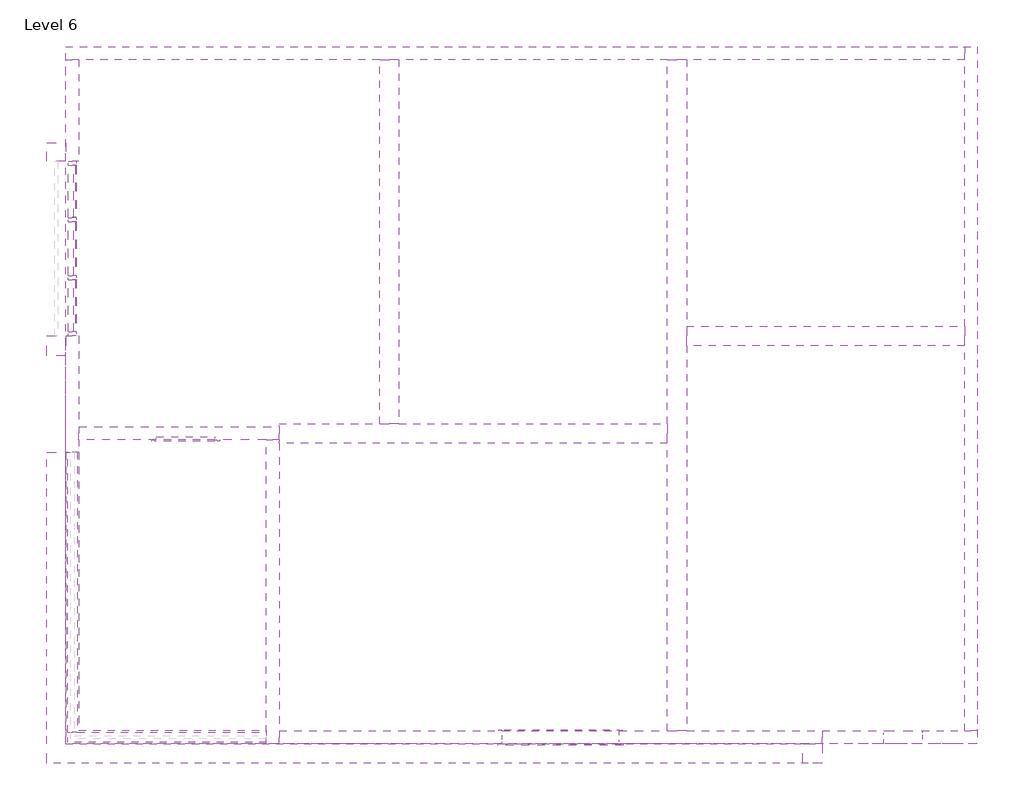
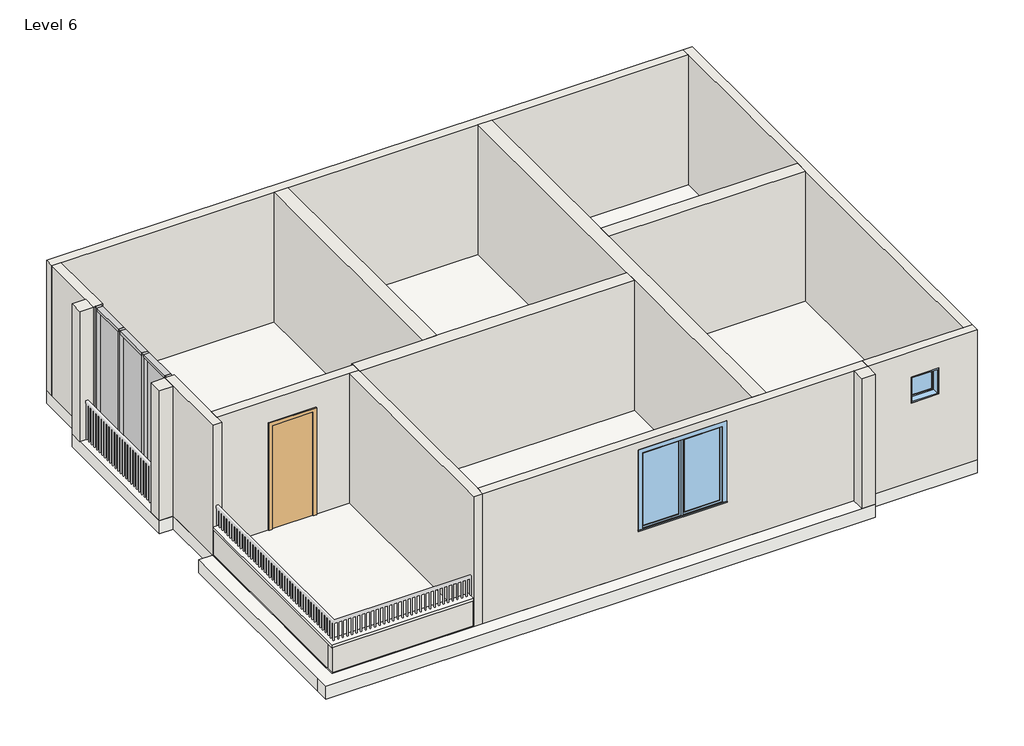
# One storey, part 1 of 2: 17 walls, 10 members, 3 plates, 3 slabs, 2 windows, 1 door.
"""IFC4 building model written with IfcOpenShell, lengths in millimetres."""

from ifc_helpers import new_model, si_unit, frame, origin, place, context, project, spatial, polyline, outline, extrude, faceted_brep, transform, mapped, element, save
from components import door_f936a269, member_eaba9652, member_3f395ae9, member_c17f1be2, member_d2e7e466, system_panel_glazed_52d31088, system_panel_glazed_f0722de2, window_97c6202a, window_6846e476

model = new_model("IFC4")

# Units and contexts
model_context = context("Model", 3, world=origin())
ifc_project = project(units=[si_unit("LENGTHUNIT", "METRE", prefix="MILLI")], contexts=[model_context])

# Site, building, storey
site = spatial("IfcSite", under=ifc_project)
building = spatial("IfcBuilding", under=site)
storey = spatial("IfcBuildingStorey", under=building, Name="Level 6", Elevation=15240.0)

# Door
placement = place(None, origin())
door_shape = door_f936a269(model_context)
element("IfcDoor", 1, ObjectType="Single-Flush : 36\" x 96\"", at=placement, inside=storey, context=model_context, shape_type="MappedRepresentation", body=[
    mapped(door_shape, transform((-16449.2169582, -4610.4617616, 16764.0), x_axis=(-1.0, 0.0, 0.0), y_axis=(0.0, -1.0, 0.0), z_axis=(0.0, 0.0, 1.0))),
])

# Members
member_shape = member_eaba9652(model_context)
element("IfcMember", 2, ObjectType="Rectangular Mullion : 2.5\" x 5\" rectangular", at=placement, inside=storey, context=model_context, shape_type="MappedRepresentation", body=[
    mapped(member_shape, transform((-18227.2169582, -1251.3117616, 16764.0), x_axis=(0.0, -1.0, 0.0), y_axis=(-1.0, 0.0, 0.0), z_axis=(0.0, 0.0, -1.0))),
])
element("IfcMember", 3, ObjectType="Rectangular Mullion : 2.5\" x 5\" rectangular", at=placement, inside=storey, context=model_context, shape_type="MappedRepresentation", body=[
    mapped(member_shape, transform((-18227.2169582, -2165.7117616, 16764.0), x_axis=(0.0, -1.0, 0.0), y_axis=(-1.0, 0.0, 0.0), z_axis=(0.0, 0.0, -1.0))),
])
member_2_shape = member_3f395ae9(model_context)
element("IfcMember", 4, ObjectType="Rectangular Mullion : 2.5\" x 5\" rectangular", at=placement, inside=storey, context=model_context, shape_type="MappedRepresentation", body=[
    mapped(member_2_shape, transform((-18227.2169582, -3080.1117616, 16764.0), x_axis=(0.0, -1.0, 0.0), y_axis=(-1.0, 0.0, 0.0), z_axis=(0.0, 0.0, -1.0))),
])
element("IfcMember", 5, ObjectType="Rectangular Mullion : 2.5\" x 5\" rectangular", at=placement, inside=storey, context=model_context, shape_type="MappedRepresentation", body=[
    mapped(member_2_shape, transform((-18227.2169582, -336.9117616, 19812.0), x_axis=(0.0, 1.0, 0.0), y_axis=(-1.0, 0.0, 0.0), z_axis=(0.0, 0.0, 1.0))),
])
member_3_shape = member_c17f1be2(model_context)
element("IfcMember", 6, ObjectType="Rectangular Mullion : 2.5\" x 5\" rectangular", at=placement, inside=storey, context=model_context, shape_type="MappedRepresentation", body=[
    mapped(member_3_shape, transform((-18227.2169582, -3016.6117616, 19812.0), x_axis=(0.0, 0.0, 1.0), y_axis=(-1.0, 0.0, 0.0), z_axis=(0.0, -1.0, 0.0))),
])
element("IfcMember", 7, ObjectType="Rectangular Mullion : 2.5\" x 5\" rectangular", at=placement, inside=storey, context=model_context, shape_type="MappedRepresentation", body=[
    mapped(member_3_shape, transform((-18227.2169582, -1219.5617616, 19812.0), x_axis=(0.0, 0.0, 1.0), y_axis=(-1.0, 0.0, 0.0), z_axis=(0.0, -1.0, 0.0))),
])
element("IfcMember", 8, ObjectType="Rectangular Mullion : 2.5\" x 5\" rectangular", at=placement, inside=storey, context=model_context, shape_type="MappedRepresentation", body=[
    mapped(member_3_shape, transform((-18227.2169582, -400.4117616, 16764.0), x_axis=(0.0, 0.0, -1.0), y_axis=(-1.0, 0.0, 0.0), z_axis=(0.0, 1.0, 0.0))),
])
element("IfcMember", 9, ObjectType="Rectangular Mullion : 2.5\" x 5\" rectangular", at=placement, inside=storey, context=model_context, shape_type="MappedRepresentation", body=[
    mapped(member_3_shape, transform((-18227.2169582, -2197.4617616, 16764.0), x_axis=(0.0, 0.0, -1.0), y_axis=(-1.0, 0.0, 0.0), z_axis=(0.0, 1.0, 0.0))),
])
member_4_shape = member_d2e7e466(model_context)
element("IfcMember", 10, ObjectType="Rectangular Mullion : 2.5\" x 5\" rectangular", at=placement, inside=storey, context=model_context, shape_type="MappedRepresentation", body=[
    mapped(member_4_shape, transform((-18227.2169582, -1283.0617616, 16764.0), x_axis=(0.0, 0.0, -1.0), y_axis=(-1.0, 0.0, 0.0), z_axis=(0.0, 1.0, 0.0))),
])
element("IfcMember", 11, ObjectType="Rectangular Mullion : 2.5\" x 5\" rectangular", at=placement, inside=storey, context=model_context, shape_type="MappedRepresentation", body=[
    mapped(member_4_shape, transform((-18227.2169582, -2133.9617616, 19812.0), x_axis=(0.0, 0.0, 1.0), y_axis=(-1.0, 0.0, 0.0), z_axis=(0.0, -1.0, 0.0))),
])

# Plates
system_panel_glazed_shape = system_panel_glazed_52d31088(model_context)
element("IfcPlate", 12, ObjectType="System Panel : Glazed", at=placement, inside=storey, context=model_context, shape_type="MappedRepresentation", body=[
    mapped(system_panel_glazed_shape, transform((-18227.2169582, -809.9867616, 16827.5), x_axis=(0.0, -1.0, 0.0), y_axis=(1.0, 0.0, 0.0), z_axis=(0.0, 0.0, 1.0))),
])
element("IfcPlate", 13, ObjectType="System Panel : Glazed", at=placement, inside=storey, context=model_context, shape_type="MappedRepresentation", body=[
    mapped(system_panel_glazed_shape, transform((-18227.2169582, -2607.0367616, 16827.5), x_axis=(0.0, -1.0, 0.0), y_axis=(1.0, 0.0, 0.0), z_axis=(0.0, 0.0, 1.0))),
])
system_panel_glazed_2_shape = system_panel_glazed_f0722de2(model_context)
element("IfcPlate", 14, ObjectType="System Panel : Glazed", at=placement, inside=storey, context=model_context, shape_type="MappedRepresentation", body=[
    mapped(system_panel_glazed_2_shape, transform((-18227.2169582, -1708.5117616, 16827.5), x_axis=(0.0, -1.0, 0.0), y_axis=(1.0, 0.0, 0.0), z_axis=(0.0, 0.0, 1.0))),
])

# Slabs
element("IfcSlab", 15, ObjectType="Generic - 12\"", at=placement, inside=storey, context=model_context, shape_type="SweptSolid", body=[
    extrude(outline(polyline([(-18633.6169582, -41.6299243), (-18328.8169582, -41.6299243), (-18328.8169582, -3394.4299243), (-18633.6169582, -3394.4299243), (-18633.6169582, -41.6299243)])), frame((0.0, 0.0, 16459.2), z_axis=(0.0, 0.0, 1.0), x_axis=(1.0, 0.0, 0.0)), (0.0, 0.0, 1.0), 304.8),
    extrude(outline(polyline([(-18633.6169582, -4908.9117616), (-18328.8169582, -4908.9117616), (-18328.8169582, -9487.2617616), (-6444.7919582, -9487.2617616), (-6444.7919582, -9792.0617616), (-18633.6169582, -9792.0617616), (-18633.6169582, -9487.2617616), (-18633.6169582, -4908.9117616)])), frame((0.0, 0.0, 16459.2), z_axis=(0.0, 0.0, 1.0), x_axis=(1.0, 0.0, 0.0)), (0.0, 0.0, 1.0), 304.8),
])
element("IfcSlab", 16, ObjectType="Generic - 12\" 2", at=placement, inside=storey, context=model_context, shape_type="SweptSolid", body=[
    extrude(outline(polyline([(-4006.3919582, 1466.4882384), (-4006.3919582, -9487.2617616), (-18328.8169582, -9487.2617616), (-18328.8169582, 1466.4882384), (-4006.3919582, 1466.4882384)])), frame((0.0, 0.0, 16459.2), z_axis=(0.0, 0.0, 1.0), x_axis=(1.0, 0.0, 0.0)), (0.0, 0.0, 1.0), 304.8),
])
element("IfcSlab", 17, ObjectType="Generic - 2\"", at=placement, inside=storey, context=model_context, shape_type="SweptSolid", body=[
    extrude(outline(polyline([(-15179.2169582, -9487.2617616), (-18328.8169582, -9487.2617616), (-18328.8169582, -4908.9117616), (-18125.6169582, -4908.9117616), (-18125.6169582, -9277.7117616), (-15179.2169582, -9277.7117616), (-15179.2169582, -9309.4617616), (-15179.2169582, -9487.2617616)])), frame((0.0, 0.0, 17373.6), z_axis=(0.0, 0.0, 1.0), x_axis=(1.0, 0.0, 0.0)), (0.0, 0.0, 1.0), 50.8),
])

# Walls
element("IfcWall", 18, ObjectType="Generic - 12\" white", at=placement, inside=storey, context=model_context, shape_type="SweptSolid", body=[
    extrude(outline(polyline([(-18633.6169582, -336.9117616), (-18633.6169582, -41.6299243), (-18328.8169582, -41.6299243), (-18328.8169582, -336.9117616), (-18633.6169582, -336.9117616)])), frame((0.0, 0.0, 16764.0), z_axis=(0.0, 0.0, 1.0), x_axis=(1.0, 0.0, 0.0)), (0.0, 0.0, 1.0), 3048.0),
])
element("IfcWall", 19, ObjectType="Generic - 12\" white", at=placement, inside=storey, context=model_context, shape_type="SweptSolid", body=[
    extrude(outline(polyline([(-18328.8169582, -3080.1117616), (-18328.8169582, -3394.4299243), (-18633.6169582, -3394.4299243), (-18633.6169582, -3080.1117616), (-18328.8169582, -3080.1117616)])), frame((0.0, 0.0, 16764.0), z_axis=(0.0, 0.0, 1.0), x_axis=(1.0, 0.0, 0.0)), (0.0, 0.0, 1.0), 3048.0),
])
element("IfcWall", 20, ObjectType="Generic - 12\" white", at=placement, inside=storey, context=model_context, shape_type="SweptSolid", body=[
    extrude(outline(polyline([(-6749.5919582, -9487.2617616), (-6444.7919582, -9487.2617616), (-6444.7919582, -9792.0617616), (-6749.5919582, -9792.0617616), (-6749.5919582, -9487.2617616)])), frame((0.0, 0.0, 16764.0), z_axis=(0.0, 0.0, 1.0), x_axis=(1.0, 0.0, 0.0)), (0.0, 0.0, 1.0), 3048.0),
])
element("IfcWall", 21, ObjectType="Generic - 12\" white", at=placement, inside=storey, context=model_context, shape_type="Brep", body=[
    faceted_brep([(-8575.2169582, -9284.0617616, 16764.0), (-8575.2169582, -3232.5117616, 16764.0), (-8575.2169582, -2927.7117616, 16764.0), (-8575.2169582, 1263.2882384, 16764.0), (-8575.2169582, 1263.2882384, 19812.0), (-8575.2169582, -2927.7117616, 19812.0), (-8575.2169582, -3232.5117616, 19812.0), (-8575.2169582, -9284.0617616, 19812.0), (-8880.0169582, -9284.0617616, 16764.0), (-8880.0169582, -9284.0617616, 19812.0), (-8880.0169582, -4762.8617616, 19812.0), (-8880.0169582, -4458.0617616, 19812.0), (-8880.0169582, 1263.2882384, 19812.0), (-8880.0169582, 1263.2882384, 16764.0), (-8880.0169582, -4458.0617616, 16764.0), (-8880.0169582, -4762.8617616, 16764.0)], [[[0, 1, 2, 3, 4, 5, 6, 7]], [[8, 9, 10, 11, 12, 13, 14, 15]], [[3, 2, 1, 0, 8, 15, 14, 13]], [[7, 6, 5, 4, 12, 11, 10, 9]], [[4, 3, 13, 12]], [[0, 7, 9, 8]]]),
])
element("IfcWall", 22, ObjectType="Generic - 12\" white", at=placement, inside=storey, context=model_context, shape_type="Brep", body=[
    faceted_brep([(-14976.0169582, -4762.8617616, 16764.0), (-8880.0169582, -4762.8617616, 16764.0), (-8880.0169582, -4762.8617616, 19812.0), (-14976.0169582, -4762.8617616, 19812.0), (-14976.0169582, -4458.0617616, 16764.0), (-14976.0169582, -4458.0617616, 19812.0), (-13401.2169582, -4458.0617616, 19812.0), (-13096.4169582, -4458.0617616, 19812.0), (-8880.0169582, -4458.0617616, 19812.0), (-8880.0169582, -4458.0617616, 16764.0), (-13096.4169582, -4458.0617616, 16764.0), (-13401.2169582, -4458.0617616, 16764.0), (-14976.0169582, -4712.0617616, 16764.0), (-14976.0169582, -4508.8617616, 16764.0), (-14976.0169582, -4508.8617616, 19812.0), (-14976.0169582, -4712.0617616, 19812.0)], [[[0, 1, 2, 3]], [[4, 5, 6, 7, 8, 9, 10, 11]], [[1, 0, 12, 13, 4, 11, 10, 9]], [[3, 2, 8, 7, 6, 5, 14, 15]], [[0, 3, 15, 14, 5, 4, 13, 12]], [[2, 1, 9, 8]]]),
])
element("IfcWall", 23, ObjectType="Generic - 12\" white", at=placement, inside=storey, context=model_context, shape_type="SweptSolid", body=[
    extrude(outline(polyline([(-13096.4169582, 1263.2882384), (-13096.4169582, -4458.0617616), (-13401.2169582, -4458.0617616), (-13401.2169582, 1263.2882384), (-13096.4169582, 1263.2882384)])), frame((0.0, 0.0, 16764.0), z_axis=(0.0, 0.0, 1.0), x_axis=(1.0, 0.0, 0.0)), (0.0, 0.0, 1.0), 3048.0),
])
element("IfcWall", 24, ObjectType="Generic - 12\" white", at=placement, inside=storey, context=model_context, shape_type="SweptSolid", body=[
    extrude(outline(polyline([(-4209.5919582, -3232.5117616), (-8575.2169582, -3232.5117616), (-8575.2169582, -2927.7117616), (-4209.5919582, -2927.7117616), (-4209.5919582, -3232.5117616)])), frame((0.0, 0.0, 16764.0), z_axis=(0.0, 0.0, 1.0), x_axis=(1.0, 0.0, 0.0)), (0.0, 0.0, 1.0), 3048.0),
])
element("IfcWall", 25, ObjectType="Generic - 6\"", at=placement, inside=storey, context=model_context, shape_type="Brep", body=[
    faceted_brep([(-15179.2169582, -9309.4617616, 16764.0), (-18151.0169582, -9309.4617616, 16764.0), (-18303.4169582, -9309.4617616, 16764.0), (-18303.4169582, -9309.4617616, 17373.6), (-18151.0169582, -9309.4617616, 17373.6), (-15179.2169582, -9309.4617616, 17373.6), (-15179.2169582, -9461.8617616, 16764.0), (-15179.2169582, -9461.8617616, 17373.6), (-18303.4169582, -9461.8617616, 17373.6), (-18303.4169582, -9461.8617616, 16764.0)], [[[0, 1, 2, 3, 4, 5]], [[6, 7, 8, 9]], [[2, 1, 0, 6, 9]], [[5, 4, 3, 8, 7]], [[0, 5, 7, 6]], [[3, 2, 9, 8]]]),
])
element("IfcWall", 26, ObjectType="Generic - 6\"", at=placement, inside=storey, context=model_context, shape_type="SweptSolid", body=[
    extrude(outline(polyline([(-18151.0169582, -4908.9117616), (-18151.0169582, -9309.4617616), (-18303.4169582, -9309.4617616), (-18303.4169582, -4908.9117616), (-18151.0169582, -4908.9117616)])), frame((0.0, 0.0, 16764.0), z_axis=(0.0, 0.0, 1.0), x_axis=(1.0, 0.0, 0.0)), (0.0, 0.0, 1.0), 609.6),
])
element("IfcWall", 27, ObjectType="Generic - 8\"", at=placement, inside=storey, context=model_context, shape_type="Brep", body=[
    faceted_brep([(-4006.3919582, -9284.0617616, 16764.0), (-4006.3919582, 1466.4882384, 16764.0), (-4006.3919582, 1466.4882384, 19812.0), (-4006.3919582, -9284.0617616, 19812.0), (-4209.5919582, -9284.0617616, 16764.0), (-4209.5919582, -9284.0617616, 19812.0), (-4209.5919582, -3232.5117616, 19812.0), (-4209.5919582, -2927.7117616, 19812.0), (-4209.5919582, 1263.2882384, 19812.0), (-4209.5919582, 1466.4882384, 19812.0), (-4209.5919582, 1466.4882384, 16764.0), (-4209.5919582, 1263.2882384, 16764.0), (-4209.5919582, -2927.7117616, 16764.0), (-4209.5919582, -3232.5117616, 16764.0)], [[[0, 1, 2, 3]], [[4, 5, 6, 7, 8, 9, 10, 11, 12, 13]], [[1, 0, 4, 13, 12, 11, 10]], [[3, 2, 9, 8, 7, 6, 5]], [[0, 3, 5, 4]], [[2, 1, 10, 9]]]),
])
element("IfcWall", 28, ObjectType="Generic - 8\"", at=placement, inside=storey, context=model_context, shape_type="Brep", body=[
    faceted_brep([(-4209.5919582, 1466.4882384, 16764.0), (-18328.8169582, 1466.4882384, 16764.0), (-18328.8169582, 1466.4882384, 19812.0), (-4209.5919582, 1466.4882384, 19812.0), (-4209.5919582, 1263.2882384, 16764.0), (-4209.5919582, 1263.2882384, 19812.0), (-8575.2169582, 1263.2882384, 19812.0), (-8880.0169582, 1263.2882384, 19812.0), (-13096.4169582, 1263.2882384, 19812.0), (-13401.2169582, 1263.2882384, 19812.0), (-18125.6169582, 1263.2882384, 19812.0), (-18328.8169582, 1263.2882384, 19812.0), (-18328.8169582, 1263.2882384, 16764.0), (-18125.6169582, 1263.2882384, 16764.0), (-13401.2169582, 1263.2882384, 16764.0), (-13096.4169582, 1263.2882384, 16764.0), (-8880.0169582, 1263.2882384, 16764.0), (-8575.2169582, 1263.2882384, 16764.0)], [[[0, 1, 2, 3]], [[4, 5, 6, 7, 8, 9, 10, 11, 12, 13, 14, 15, 16, 17]], [[1, 0, 4, 17, 16, 15, 14, 13, 12]], [[3, 2, 11, 10, 9, 8, 7, 6, 5]], [[0, 3, 5, 4]], [[2, 1, 12, 11]]]),
])
element("IfcWall", 29, ObjectType="Generic - 8\"", at=placement, inside=storey, context=model_context, shape_type="SweptSolid", body=[
    extrude(outline(polyline([(-18328.8169582, -336.9117616), (-18328.8169582, 1263.2882384), (-18125.6169582, 1263.2882384), (-18125.6169582, -336.9117616), (-18328.8169582, -336.9117616)])), frame((0.0, 0.0, 16764.0), z_axis=(0.0, 0.0, 1.0), x_axis=(1.0, 0.0, 0.0)), (0.0, 0.0, 1.0), 3048.0),
])
element("IfcWall", 30, ObjectType="Generic - 8\"", at=placement, inside=storey, context=model_context, shape_type="Brep", body=[
    faceted_brep([(-18328.8169582, -3080.1117616, 16764.0), (-18328.8169582, -4908.9117616, 16764.0), (-18328.8169582, -4908.9117616, 19812.0), (-18328.8169582, -3080.1117616, 19812.0), (-18125.6169582, -3080.1117616, 16764.0), (-18125.6169582, -3080.1117616, 19812.0), (-18125.6169582, -4508.8617616, 19812.0), (-18125.6169582, -4712.0617616, 19812.0), (-18125.6169582, -4908.9117616, 19812.0), (-18125.6169582, -4908.9117616, 16764.0), (-18125.6169582, -4712.0617616, 16764.0), (-18125.6169582, -4508.8617616, 16764.0), (-18151.0169582, -4908.9117616, 16764.0), (-18303.4169582, -4908.9117616, 16764.0)], [[[0, 1, 2, 3]], [[4, 5, 6, 7, 8, 9, 10, 11]], [[1, 0, 4, 11, 10, 9, 12, 13]], [[2, 1, 13, 12, 9, 8]], [[3, 2, 8, 7, 6, 5]], [[0, 3, 5, 4]]]),
])
element("IfcWall", 31, ObjectType="Generic - 8\" 2", at=placement, inside=storey, context=model_context, shape_type="Brep", body=[
    faceted_brep([(-4006.3919582, -9284.0617616, 16764.0), (-4209.5919582, -9284.0617616, 16764.0), (-6444.7919582, -9284.0617616, 16764.0), (-6444.7919582, -9284.0617616, 19812.0), (-4209.5919582, -9284.0617616, 19812.0), (-4006.3919582, -9284.0617616, 19812.0), (-4869.9919582, -9284.0617616, 19220.2087386), (-5479.5919582, -9284.0617616, 19220.2087386), (-5479.5919582, -9284.0617616, 18610.6087386), (-4869.9919582, -9284.0617616, 18610.6087386), (-4006.3919582, -9487.2617616, 16764.0), (-4006.3919582, -9487.2617616, 19812.0), (-6444.7919582, -9487.2617616, 19812.0), (-6444.7919582, -9487.2617616, 16764.0), (-4869.9919582, -9487.2617616, 19220.2087386), (-4869.9919582, -9487.2617616, 18610.6087386), (-5479.5919582, -9487.2617616, 18610.6087386), (-5479.5919582, -9487.2617616, 19220.2087386)], [[[0, 1, 2, 3, 4, 5], [6, 7, 8, 9]], [[10, 11, 12, 13], [14, 15, 16, 17]], [[2, 1, 0, 10, 13]], [[3, 2, 13, 12]], [[5, 4, 3, 12, 11]], [[0, 5, 11, 10]], [[15, 14, 6, 9]], [[16, 15, 9, 8]], [[17, 16, 8, 7]], [[14, 17, 7, 6]]]),
])
element("IfcWall", 32, ObjectType="Generic - 8\" 3", at=placement, inside=storey, context=model_context, shape_type="Brep", body=[
    faceted_brep([(-14976.0169582, -4712.0617616, 19812.0), (-15179.2169582, -4712.0617616, 19812.0), (-18125.6169582, -4712.0617616, 19812.0), (-18125.6169582, -4712.0617616, 16764.0), (-16906.4169582, -4712.0617616, 16764.0), (-16906.4169582, -4712.0617616, 19202.4), (-15992.0169582, -4712.0617616, 19202.4), (-15992.0169582, -4712.0617616, 16764.0), (-15179.2169582, -4712.0617616, 16764.0), (-14976.0169582, -4712.0617616, 16764.0), (-18125.6169582, -4508.8617616, 19812.0), (-14976.0169582, -4508.8617616, 19812.0), (-14976.0169582, -4508.8617616, 16764.0), (-15992.0169582, -4508.8617616, 16764.0), (-15992.0169582, -4508.8617616, 19202.4), (-16906.4169582, -4508.8617616, 19202.4), (-16906.4169582, -4508.8617616, 16764.0), (-18125.6169582, -4508.8617616, 16764.0)], [[[0, 1, 2, 3, 4, 5, 6, 7, 8, 9]], [[10, 11, 12, 13, 14, 15, 16, 17]], [[3, 17, 16, 4]], [[12, 9, 8, 7, 13]], [[2, 1, 0, 11, 10]], [[3, 2, 10, 17]], [[0, 9, 12, 11]], [[15, 5, 4, 16]], [[5, 15, 14, 6]], [[6, 14, 13, 7]]]),
])
element("IfcWall", 33, ObjectType="Generic - 8\" 3", at=placement, inside=storey, context=model_context, shape_type="Brep", body=[
    faceted_brep([(-15179.2169582, -4712.0617616, 16764.0), (-15179.2169582, -9309.4617616, 16764.0), (-15179.2169582, -9461.8617616, 16764.0), (-15179.2169582, -9487.2617616, 16764.0), (-15179.2169582, -9487.2617616, 19812.0), (-15179.2169582, -4712.0617616, 19812.0), (-14976.0169582, -4712.0617616, 16764.0), (-14976.0169582, -4712.0617616, 19812.0), (-14976.0169582, -4762.8617616, 19812.0), (-14976.0169582, -9284.0617616, 19812.0), (-14976.0169582, -9487.2617616, 19812.0), (-14976.0169582, -9487.2617616, 16764.0), (-14976.0169582, -9284.0617616, 16764.0), (-14976.0169582, -4762.8617616, 16764.0)], [[[0, 1, 2, 3, 4, 5]], [[6, 7, 8, 9, 10, 11, 12, 13]], [[3, 2, 1, 0, 6, 13, 12, 11]], [[5, 4, 10, 9, 8, 7]], [[0, 5, 7, 6]], [[3, 11, 10, 4]]]),
])
element("IfcWall", 34, ObjectType="Generic - 8\" 3", at=placement, inside=storey, context=model_context, shape_type="Brep", body=[
    faceted_brep([(-6444.7919582, -9284.0617616, 16764.0), (-8575.2169582, -9284.0617616, 16764.0), (-8880.0169582, -9284.0617616, 16764.0), (-14976.0169582, -9284.0617616, 16764.0), (-14976.0169582, -9284.0617616, 19812.0), (-8880.0169582, -9284.0617616, 19812.0), (-8575.2169582, -9284.0617616, 19812.0), (-6444.7919582, -9284.0617616, 19812.0), (-11470.8169582, -9284.0617616, 19562.2375963), (-11470.8169582, -9284.0617616, 17733.4375963), (-9642.0169582, -9284.0617616, 17733.4375963), (-9642.0169582, -9284.0617616, 19562.2375963), (-6444.7919582, -9487.2617616, 16764.0), (-6444.7919582, -9487.2617616, 19812.0), (-14976.0169582, -9487.2617616, 19812.0), (-14976.0169582, -9487.2617616, 16764.0), (-11470.8169582, -9487.2617616, 19562.2375963), (-9642.0169582, -9487.2617616, 19562.2375963), (-9642.0169582, -9487.2617616, 17733.4375963), (-11470.8169582, -9487.2617616, 17733.4375963)], [[[0, 1, 2, 3, 4, 5, 6, 7], [8, 9, 10, 11]], [[12, 13, 14, 15], [16, 17, 18, 19]], [[3, 2, 1, 0, 12, 15]], [[7, 6, 5, 4, 14, 13]], [[0, 7, 13, 12]], [[3, 15, 14, 4]], [[9, 8, 16, 19]], [[10, 9, 19, 18]], [[11, 10, 18, 17]], [[8, 11, 17, 16]]]),
])

# Windows
window_shape = window_97c6202a(model_context)
element("IfcWindow", 35, ObjectType="Casement Dbl with Trim.0001 : 72\" x 72\"", at=placement, inside=storey, context=model_context, shape_type="MappedRepresentation", body=[
    mapped(window_shape, transform((-10556.4169582, -9366.6117616, 16819.0375963), x_axis=(-1.0, 0.0, 0.0), y_axis=(0.0, -1.0, 0.0), z_axis=(0.0, 0.0, 1.0))),
])
window_2_shape = window_6846e476(model_context)
element("IfcWindow", 36, ObjectType="Fixed : 24\" x 24\"", at=placement, inside=storey, context=model_context, shape_type="MappedRepresentation", body=[
    mapped(window_2_shape, transform((-5136.6919582, -9385.6617616, 17696.2087386), x_axis=(1.0, 0.0, 0.0), y_axis=(0.0, 1.0, 0.0), z_axis=(0.0, 0.0, 1.0))),
])

save(model, "model.ifc")

# Revit data of these elements
# Type "Single-Flush : 36\" x 96\""
#   Type Mark = "1"
#   Construction Type Id = "MDOOR"
#   Assembly Code = "C1020"
#   Analytic Construction = "Metal"
#   Thickness = 0' - 2"
#   Heat Transfer Coefficient (U) = 0.651978 BTU/(h·ft²·°F)
#   Height = 8' - 0"
#   Trim Projection Ext = 0' - 1"
#   Trim Projection Int = 0' - 1"
#   Trim Width = 0' - 3"
#   Width = 3' - 0"
#   Define Thermal Properties by = 1
#   Door Material = Glass, Clear Glazing
#   Frame Material = Iron, Ductile
#   Visual Light Transmittance = 0
#   Solar Heat Gain Coefficient = 0
#   Function = (empty or 0)
#   Wall Closure = (empty or 0)
# Type "Rectangular Mullion : 2.5\" x 5\" rectangular"
#   built-in parameter 1007304 = 0.416667 (stored number, unit not read)
#   built-in parameter 1007301 = 0.104167 (stored number, unit not read)
#   built-in parameter 1007300 = 0.104167 (stored number, unit not read)
# Type "System Panel : Glazed"
#   Construction Type Id = "GSP4R"
#   Analytic Construction = "1/8 in Pilkington single glazing"
#   Visual Light Transmittance = 0.9
#   Solar Heat Gain Coefficient = 0.86
#   Heat Transfer Coefficient (U) = 1.18115 BTU/(h·ft²·°F)
# Type "Generic - 12\""
#   Assembly Code = "B1010"
#   Function = 0
#   Layers, outside or top first: 1' - 0" "Parking Stripe" (function 1)
# Type "Generic - 12\" 2"
#   Assembly Code = "B1010"
#   Function = 0
#   Layers, outside or top first: 1' - 0" "Parking Stripe" (function 1)
# Type "Generic - 2\""
#   Assembly Code = "B1010"
#   Function = 0
#   Layers, outside or top first: 0' - 2" "Parking Stripe" (function 1)
# Type "Generic - 12\" white"
#   Assembly Code = "B2010"
#   Layers, outside or top first: 1' - 0" "Parking Stripe" (function 1)
# Type "Generic - 6\""
#   Assembly Code = "B2010"
#   Layers, outside or top first: 0' - 6" "Concrete Masonry Units" (function 1)
# Type "Generic - 8\""
#   Assembly Code = "B2010"
#   Layers, outside or top first: 0' - 8" "Door - Frame" (function 1)
# Type "Generic - 8\" 2"
#   Assembly Code = "B2010"
#   Layers, outside or top first: 0' - 8" "Door - Frame" (function 1)
# Type "Generic - 8\" 3"
#   Assembly Code = "B2010"
#   Layers, outside or top first: 0' - 8" "EIFS, Exterior Insulation" (function 1)
# Type "Casement Dbl with Trim.0001 : 72\" x 72\""
#   Type Mark = "10"
#   Construction Type Id = "GSP4R"
#   Assembly Code = "B2020100"
#   Analytic Construction = "1/8 in Pilkington single glazing"
#   Visual Light Transmittance = 0.9
#   Solar Heat Gain Coefficient = 0.78
#   Heat Transfer Coefficient (U) = 0.6496 BTU/(h·ft²·°F)
#   Height = 6' - 0"
#   Default Sill Height = 3' - 0"
#   Trim Projection - Ext. = 0' - 0 1/2"
#   Trim Projection - Int. = 0' - 0 3/4"
#   Trim Width - Exterior = 0' - 3 1/2"
#   Trim Width - Interior = 0' - 3 1/2"
#   Width = 6' - 0"
#   Window Inset = 0' - 0 3/4"
#   Define Thermal Properties by = 1
#   Glass Pane Material = Glass
#   Sash Material = Iron, Ductile
#   Trim Exterior Material = Iron, Ductile
#   Trim Interior Material = Iron, Ductile
#   Wall Closure = (empty or 0)
# Type "Fixed : 24\" x 24\""
#   Type Mark = "3"
#   Construction Type Id = "GSP4R"
#   Assembly Code = "B2020100"
#   Analytic Construction = "1/8 in Pilkington single glazing"
#   Visual Light Transmittance = 0.9
#   Solar Heat Gain Coefficient = 0.78
#   Heat Transfer Coefficient (U) = 0.6496 BTU/(h·ft²·°F)
#   Height = 2' - 0"
#   Default Sill Height = 3' - 0"
#   Width = 2' - 0"
#   Window Inset = 0' - 0 3/4"
#   Define Thermal Properties by = 1
#   Glass Pane Material = Glass
#   Sash Material = Iron, Ductile
#   Wall Closure = (empty or 0)
# Element 1 (IfcDoor, "Single-Flush : 36\" x 96\"")
#   Phase Created = New Construction
#   Materials on its faces: "Iron, Ductile", "Glass, Clear Glazing"
# Elements 2, 3, 4, 5, 6, 7, 8, 9, 10, 11 (IfcMember, "Rectangular Mullion : 2.5\" x 5\" rectangular")
#   Phase Created = New Construction
#   Materials on its faces: "Iron, Ductile"
# Elements 12, 13, 14 (IfcPlate, "System Panel : Glazed")
#   Phase Created = New Construction
#   Materials on its faces: "Glass"
# Element 15 (IfcSlab, "Generic - 12\"")
#   built-in parameter 1001955 = 3.14159 (stored number, unit not read)
#   Height Offset From Level = 5' - 0"
#   Phase Created = New Construction
#   Materials on its faces: "Parking Stripe"
# Element 16 (IfcSlab, "Generic - 12\" 2")
#   Height Offset From Level = 5' - 0"
#   Phase Created = New Construction
#   Materials on its faces: "Parking Stripe"
# Element 17 (IfcSlab, "Generic - 2\"")
#   built-in parameter 1001955 = -1.5708 (stored number, unit not read)
#   Height Offset From Level = 7' - 2"
#   Phase Created = New Construction
#   Materials on its faces: "Parking Stripe"
# Elements 18, 19, 20, 21, 22, 23, 24 (IfcWall, "Generic - 12\" white")
#   built-in parameter 1001111 = 5' - 0"
#   Top Offset = 0' - 0"
#   Base Offset = 5' - 0"
#   Unconnected Height = 10' - 0"
#   wall height = 10' - 0"
#   Phase Created = New Construction
#   Base Constraint = Level 6
#   Materials on its faces: "Parking Stripe"
# Elements 25, 26 (IfcWall, "Generic - 6\"")
#   built-in parameter 1001111 = 5' - 0"
#   Top Offset = 0' - 0"
#   Base Offset = 5' - 0"
#   Unconnected Height = 2' - 0"
#   wall height = 2' - 0"
#   Phase Created = New Construction
#   Base Constraint = Level 6
#   Materials on its faces: "Concrete Masonry Units"
# Elements 27, 28, 29, 30 (IfcWall, "Generic - 8\"")
#   built-in parameter 1001111 = 5' - 0"
#   Top Offset = 0' - 0"
#   Base Offset = 5' - 0"
#   Unconnected Height = 10' - 0"
#   wall height = 10' - 0"
#   Phase Created = New Construction
#   Base Constraint = Level 6
#   Materials on its faces: "Door - Frame"
# Element 31 (IfcWall, "Generic - 8\" 2")
#   built-in parameter 1001111 = 5' - 0"
#   Top Offset = 0' - 0"
#   Base Offset = 5' - 0"
#   Unconnected Height = 10' - 0"
#   wall height = 10' - 0"
#   Phase Created = New Construction
#   Base Constraint = Level 6
#   Materials on its faces: "Door - Frame"
# Elements 32, 33, 34 (IfcWall, "Generic - 8\" 3")
#   built-in parameter 1001111 = 5' - 0"
#   Top Offset = 0' - 0"
#   Base Offset = 5' - 0"
#   Unconnected Height = 10' - 0"
#   wall height = 10' - 0"
#   Phase Created = New Construction
#   Base Constraint = Level 6
#   Materials on its faces: "EIFS, Exterior Insulation"
# Element 35 (IfcWindow, "Casement Dbl with Trim.0001 : 72\" x 72\"")
#   Mark = "10"
#   Phase Created = New Construction
#   Materials on its faces: "Iron, Ductile", "Glass"
# Element 36 (IfcWindow, "Fixed : 24\" x 24\"")
#   Mark = "9"
#   Phase Created = New Construction
#   Materials on its faces: "Iron, Ductile", "Glass"
# Materials
#   "Glass, Clear Glazing": class "Glass", colour RGB 0 128 192, transparency 0.75, Description = "Clear glazing", Cost = 0
#   "Iron, Ductile": class "Metal", colour RGB 0 0 0, transparency 0, Description = "Ductile cast iron", Cost = 0
#   "Parking Stripe": class "Paint", colour RGB 250 250 91, transparency 0, Cost = 0
#   "Concrete Masonry Units": class "Masonry", colour RGB 227 227 227, transparency 0, Description = "Concrete masonry units", Cost = 0
#   "Door - Frame": colour RGB 118 70 51, transparency 0, Cost = 0
#   "EIFS, Exterior Insulation": class "Generic", colour RGB 127 127 127, transparency 0, Description = "EIFS - Exterior Insulation", Cost = 0
#   "Glass": class "Glass", colour RGB 0 128 192, transparency 0.75, Description = "Soda Lime Glass", Cost = 0
